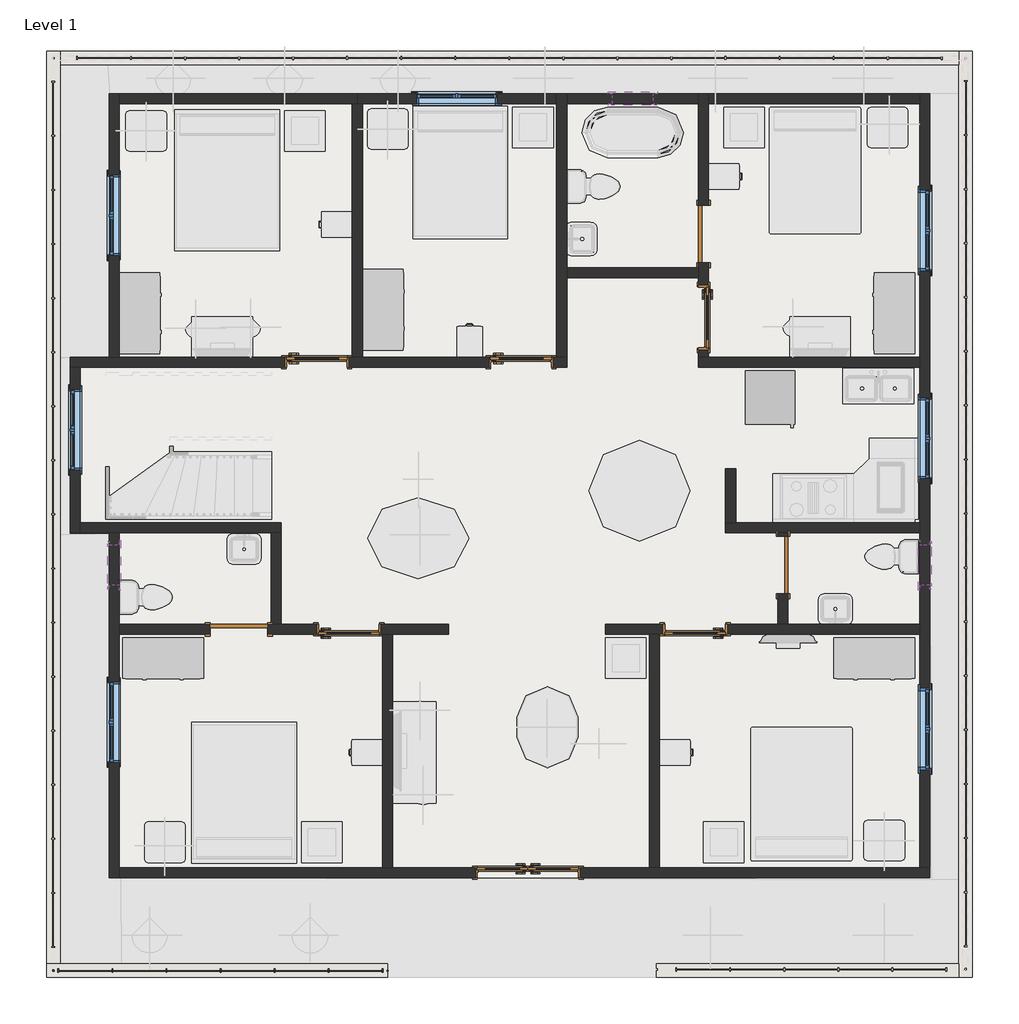
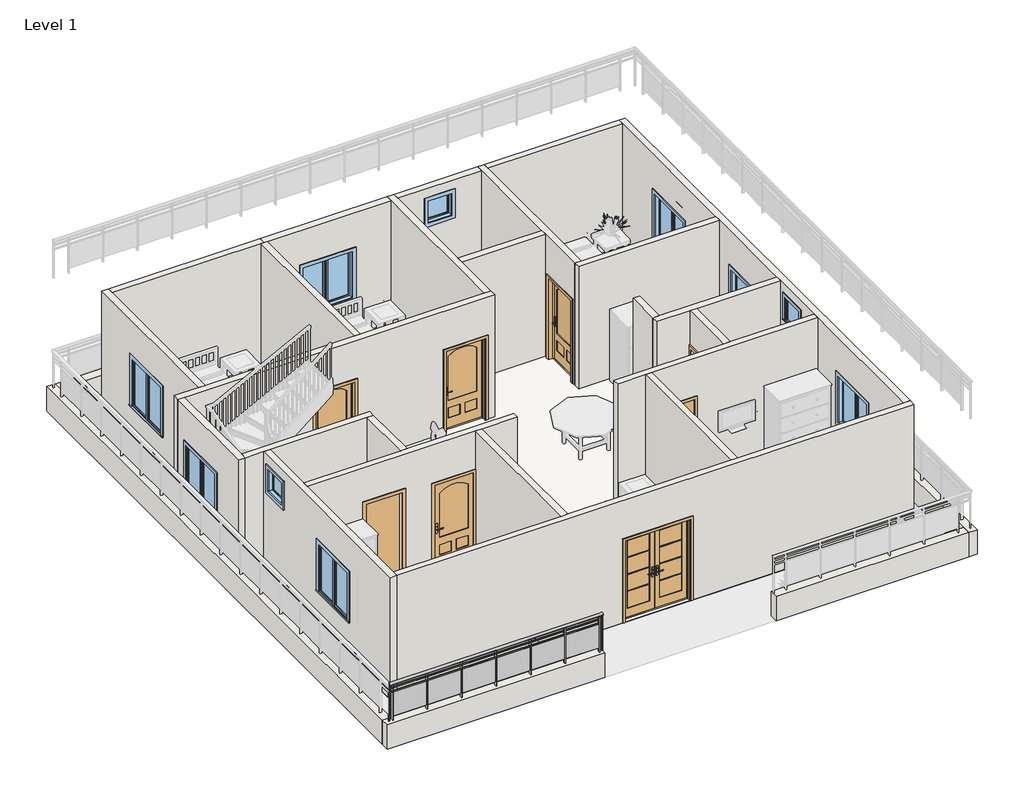
# One storey, part 1 of 5: 29 walls, 10 windows, 9 doors, 1 railing, 1 slab.
# Revit data of these elements (continued)
# Room at (-4602.324, 4275.914) mm, phase "New Construction", upper level "Level 1", upper offset 10' - 0", lower offset 0' - 0"
#   Number = "11"
#   Name = "LIVING/DRAWING AREA"
# Room at (-8722.56, 11744.633) mm, phase "New Construction", upper level "Level 1", upper offset 10' - 0", lower offset 0' - 0"
#   Number = "1"
#   Name = "BEDROOM-1"
# Room at (-5531.202, 11744.633) mm, phase "New Construction", upper level "Level 1", upper offset 10' - 0", lower offset 0' - 0"
#   Number = "2"
#   Name = "BEDROOM-2"
# Room at (-2839.36, 12577.161) mm, phase "New Construction", upper level "Level 1", upper offset 10' - 0", lower offset 0' - 0"
#   Number = "3"
# Room at (0, 11744.633) mm, phase "New Construction", upper level "Level 1", upper offset 10' - 0", lower offset 0' - 0"
#   Number = "4"
#   Name = "BEDROOM-3"
# Room at (-9399.201, 6453.241) mm, phase "New Construction", upper level "Level 1", upper offset 10' - 0", lower offset 0' - 0"
#   Number = "5"
# Room at (-8527.348, 3303.856) mm, phase "New Construction", upper level "Level 1", upper offset 10' - 0", lower offset 0' - 0"
#   Number = "6"
#   Name = "BEDROOM-4"
# Room at (-362.44, 3726.487) mm, phase "New Construction", upper level "Level 1", upper offset 10' - 0", lower offset 0' - 0"
#   Number = "7"
#   Name = "BEDROOM-5"
# Room at (568.327, 6453.241) mm, phase "New Construction", upper level "Level 1", upper offset 10' - 0", lower offset 0' - 0"
#   Number = "8"
